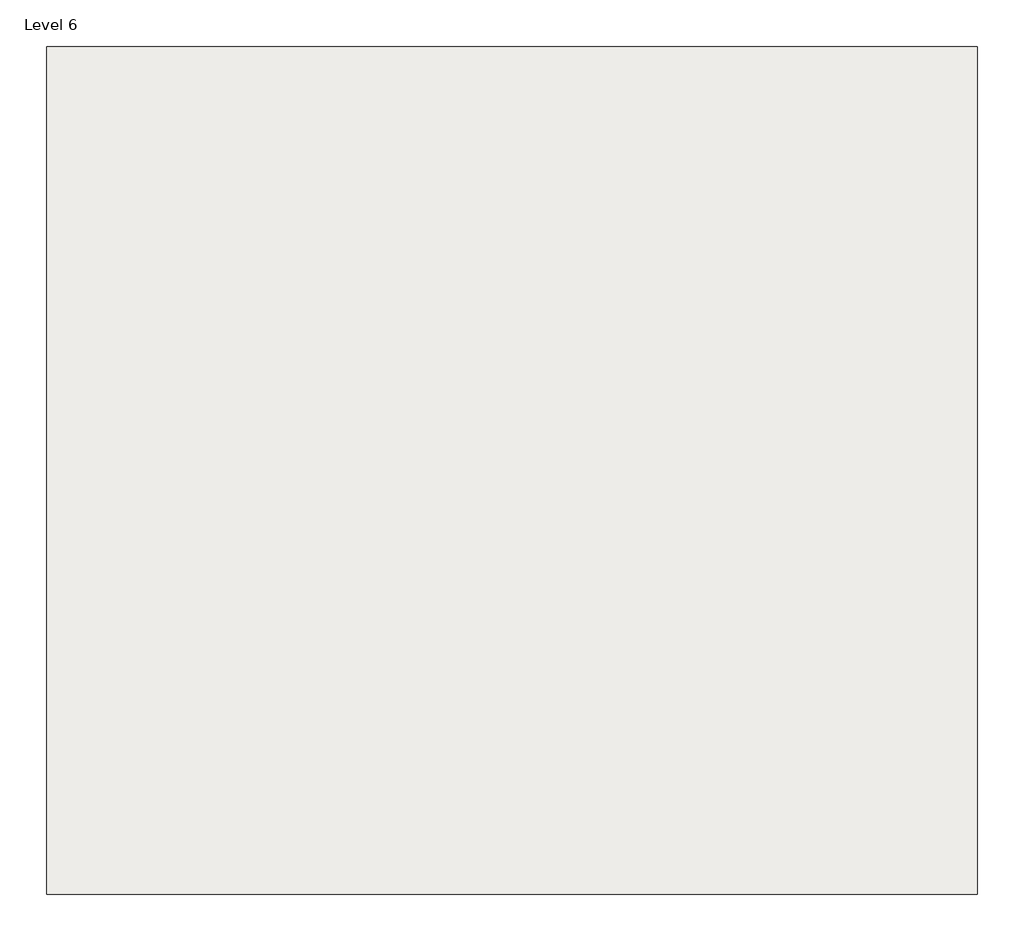
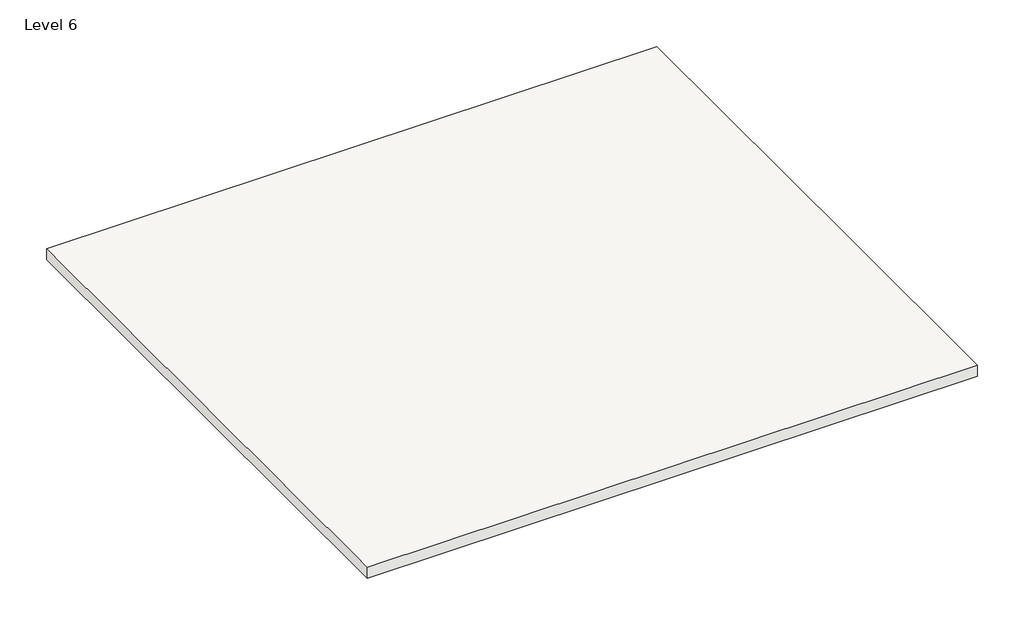
# One storey: 1 roof.
"""IFC4 building model written with IfcOpenShell, lengths in millimetres."""

from ifc_helpers import new_model, si_unit, frame, origin, place, context, project, spatial, polyline, outline, extrude, element, save

model = new_model("IFC4")

# Units and contexts
model_context = context("Model", 3, world=origin())
ifc_project = project(units=[si_unit("LENGTHUNIT", "METRE", prefix="MILLI")], contexts=[model_context])

# Site, building, storey
site = spatial("IfcSite", under=ifc_project)
building = spatial("IfcBuilding", under=site)
storey = spatial("IfcBuildingStorey", under=building, Name="Level 6", Elevation=18288.0)

# Roof
placement = place(None, origin())
element("IfcRoof", 1, ObjectType="Generic - 12\"", at=placement, inside=storey, context=model_context, shape_type="SweptSolid", body=[
    extrude(outline(polyline([(-9379.3749149, 10724.4481987), (6775.0250851, 10724.4481987), (6775.0250851, 1831.4548743), (6775.0250851, -3982.1518013), (-9379.3749149, -3982.1518013), (-9379.3749149, 10724.4481987)])), frame((0.0, 0.0, 18288.0), z_axis=(0.0, 0.0, 1.0), x_axis=(1.0, 0.0, 0.0)), (0.0, 0.0, 1.0), 304.8),
])

save(model, "model.ifc")

# Revit data of these elements
# Type "Generic - 12\""
#   Assembly Code = "B1020"
#   Layers, outside or top first: 1' - 0" no material (function 1)
# Element 1 (IfcRoof, "Generic - 12\"")
#   built-in parameter 1001705 = 61 (stored number, unit not read)
#   built-in parameter 1001710 = 33615
#   Phase Created = New Construction
#   Materials on its faces: "Default Roof"
# Materials
#   "Default Roof": colour RGB 88 101 114, transparency 0
